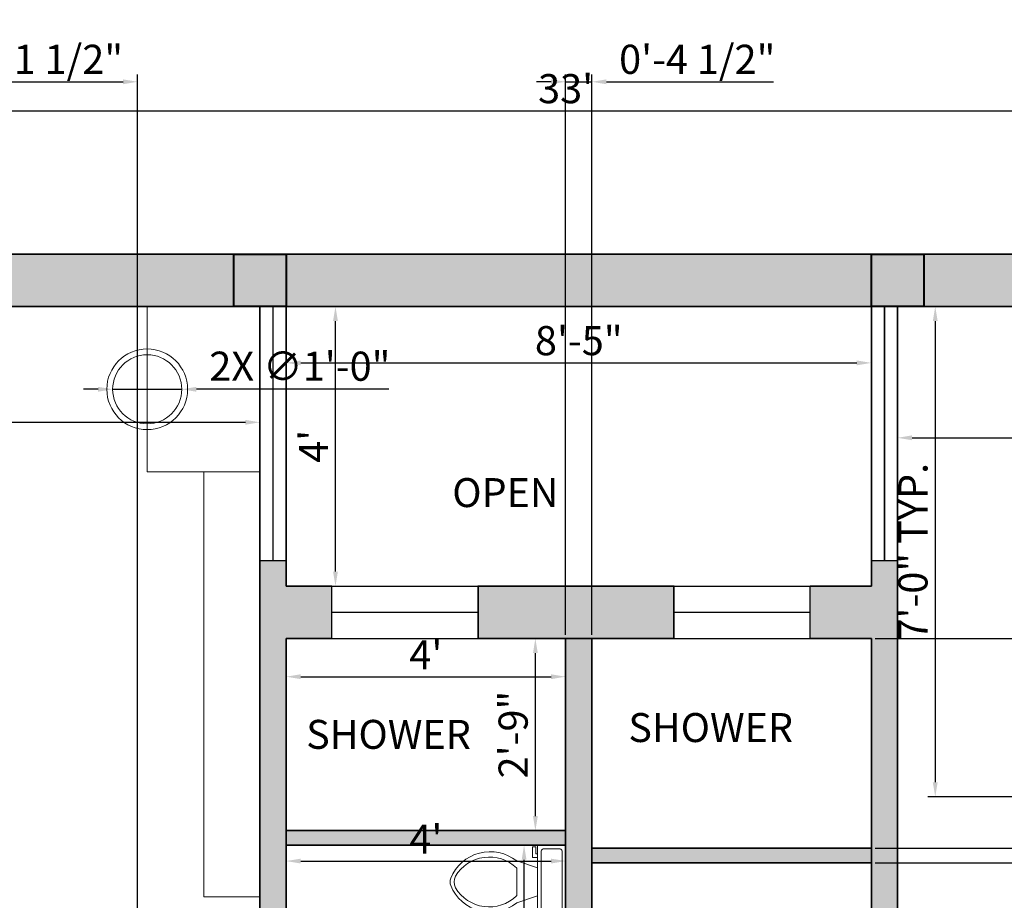
# Model space of a CAD drawing. Units: inches. Extents: x 1674 to 2231, y 1328 to 1959.
# Tile 5 of 6: x 1841 to 2010, y 1807 to 1959. Entities that reach past the tile are written whole.
import ezdxf

# ---------------------------------------------------------------- set-up
doc = ezdxf.new("R2010")
doc.units = ezdxf.units.IN
for name, color, linetype, lineweight in [('A-ANNO-DIMS', 113, 'Continuous', 18), ('A-AREA-IDEN', 113, 'Continuous', 18), ('A-COLS-PATT', 10, 'Continuous', 13), ('A-FLOR-CASE', 211, 'Continuous', 18), ('A-FLOR-FIXT', 211, 'Continuous', 18), ('A-WALL-PATT', 140, 'Continuous', 13), ('COLUMN', 10, 'Continuous', 40), ('FUR', 211, 'Continuous', 18), ('WALL', 7, 'Continuous', 35), ('WN', 181, 'Continuous', 25)]:
    doc.layers.add(name, color=color, linetype=linetype, lineweight=lineweight)
doc.styles.get("Standard").update_dxf_attribs({"font": 'arial.ttf'})
doc.dimstyles.new('ISO-25', dxfattribs={"dimtxt": 5, "dimasz": 2.5, "dimexe": 1.25, "dimexo": 0.625, "dimtad": 1, "dimdec": 0, "dimlunit": 4, "dimtxsty": 'Standard', "dimcen": 2.5, "dimadec": 0, "dimazin": 0, "dimtfac": 1, "dimtdec": 0, "dimtmove": 0, "dimatfit": 3, "dimfxl": 1, "dimarcsym": 0})

# ---------------------------------------------------------------- blocks, each defined once
blk = doc.blocks.new('*U4')
for p, q in [((9.5, -6), (9.5, -2)), ((-8, -8.5), (-8, -8)), ((-7, -8), (-7, -9.5)), ((-4, -8), (-6, -14)), ((4, -8), (6, -14)), ((-10, -8.5), (-8, -8.5)), ((-10, -9.5), (-10, -8.5)), ((-7, -9.5), (-10, -9.5)), ((4, -14), (-4, -14))]:
    blk.add_line(p, q)
blk.add_lwpolyline([(10.5, -8), (10.5, 0), (-10.5, 0), (-10.5, -8)], close=True)
for points in [[(-9.5, -2), (-9.5, -6)], [(8.5, -1), (-8.5, -1)], [(-8.5, -7), (8.5, -7)]]:
    blk.add_lwpolyline(points)
for centre, radius, start, end in [((-8.62, -1.88), 0.884, 81.8699, 188.1301), ((8.62, -1.88), 0.884, 351.8699, 98.1301), ((-8.62, -6.12), 0.884, 171.8699, 278.1301), ((8.62, -6.12), 0.884, 261.8699, 8.1301), ((3.52, -21.58), 12.17, 141.4691, 247.9714), ((4.2, -21.82), 11.33, 136.3677, 238.9468), ((-3.52, -21.58), 12.17, 292.0284, 38.5307), ((-4.2, -21.82), 11.33, 301.053, 43.6321), ((0, -27.88), 4, 245.7318, 294.2682), ((0, -29), 4, 254.8605, 285.1395)]:
    blk.add_arc(centre, radius, start, end)
blk = doc.blocks.new('*D9')
at = {"layer": 'A-ANNO-DIMS', "color": 0, "lineweight": -2, "transparency": 16777216}
for p, q in [((1736.27, 1918.98), (1736.27, 1944.21)), ((1738.77, 1942.96), (2129.77, 1942.96)), ((2132.27, 1918.98), (2132.27, 1944.21))]:
    blk.add_line(p, q, dxfattribs=at)
at = {"layer": 'A-ANNO-DIMS', "color": 0, "lineweight": 100, "transparency": 16777216}
for points in [[(1738.77, 1943.37), (1738.77, 1942.54), (1736.27, 1942.96)], [(2129.77, 1943.37), (2129.77, 1942.54), (2132.27, 1942.96)]]:
    blk.add_solid(points, dxfattribs=at)
at = {"layer": 'Defpoints', "color": 0, "lineweight": 100, "transparency": 16777216}
for p in [(2132.27, 1942.96), (1736.27, 1918.36), (2132.27, 1918.36)]:
    blk.add_point(p, dxfattribs=at)
at = {"layer": 'A-ANNO-DIMS', "color": 0, "transparency": 16777216, "insert": (1934.27, 1946.13), "char_height": 5, "attachment_point": 5}
blk.add_mtext("33'", dxfattribs=at)
blk = doc.blocks.new('*D11')
at = {"layer": 'A-ANNO-DIMS', "color": 0, "lineweight": -2, "transparency": 16777216}
for p, q in [((1745.27, 1908.73), (1745.27, 1888.23)), ((1881.77, 1908.73), (1881.77, 1888.23)), ((1747.77, 1889.48), (1879.27, 1889.48))]:
    blk.add_line(p, q, dxfattribs=at)
at = {"layer": 'A-ANNO-DIMS', "color": 0, "lineweight": 100, "transparency": 16777216}
for points in [[(1747.77, 1889.9), (1747.77, 1889.07), (1745.27, 1889.48)], [(1879.27, 1889.9), (1879.27, 1889.07), (1881.77, 1889.48)]]:
    blk.add_solid(points, dxfattribs=at)
at = {"layer": 'Defpoints', "color": 0, "lineweight": 100, "transparency": 16777216}
for p in [(1745.27, 1909.36), (1881.77, 1909.36), (1881.77, 1889.48)]:
    blk.add_point(p, dxfattribs=at)
at = {"layer": 'A-ANNO-DIMS', "color": 0, "transparency": 16777216, "insert": (1813.52, 1892.66), "char_height": 5, "attachment_point": 5}
blk.add_mtext('11\'-5"', dxfattribs=at)
blk = doc.blocks.new('*D13')
at = {"layer": 'A-ANNO-DIMS', "color": 0, "lineweight": -2, "transparency": 16777216}
for p, q in [((1886.27, 1908.73), (1886.27, 1898.44)), ((1986.77, 1908.73), (1986.77, 1898.44)), ((1888.77, 1899.69), (1984.27, 1899.69))]:
    blk.add_line(p, q, dxfattribs=at)
at = {"layer": 'A-ANNO-DIMS', "color": 0, "lineweight": 100, "transparency": 16777216}
for points in [[(1888.77, 1900.1), (1888.77, 1899.27), (1886.27, 1899.69)], [(1984.27, 1900.1), (1984.27, 1899.27), (1986.77, 1899.69)]]:
    blk.add_solid(points, dxfattribs=at)
at = {"layer": 'Defpoints', "color": 0, "lineweight": 100, "transparency": 16777216}
for p in [(1886.27, 1909.36), (1986.77, 1909.36), (1986.77, 1899.69)]:
    blk.add_point(p, dxfattribs=at)
at = {"layer": 'A-ANNO-DIMS', "color": 0, "transparency": 16777216, "insert": (1936.52, 1902.86), "char_height": 5, "attachment_point": 5}
blk.add_mtext('8\'-5"', dxfattribs=at)
blk = doc.blocks.new('*D14')
at = {"layer": 'A-ANNO-DIMS', "color": 0, "lineweight": -2, "transparency": 16777216}
for p, q in [((1886.9, 1909.36), (1895.99, 1909.36)), ((1894.74, 1863.86), (1894.74, 1906.86)), ((1886.9, 1861.36), (1895.99, 1861.36))]:
    blk.add_line(p, q, dxfattribs=at)
at = {"layer": 'A-ANNO-DIMS', "color": 0, "lineweight": 100, "transparency": 16777216}
for points in [[(1894.32, 1906.86), (1895.16, 1906.86), (1894.74, 1909.36)], [(1894.32, 1863.86), (1895.16, 1863.86), (1894.74, 1861.36)]]:
    blk.add_solid(points, dxfattribs=at)
at = {"layer": 'Defpoints', "color": 0, "lineweight": 100, "transparency": 16777216}
for p in [(1886.27, 1909.36), (1894.74, 1909.36), (1886.27, 1861.36)]:
    blk.add_point(p, dxfattribs=at)
at = {"layer": 'A-ANNO-DIMS', "color": 0, "transparency": 16777216, "insert": (1891.61, 1885.36), "char_height": 5, "attachment_point": 5, "rotation": 90}
blk.add_mtext("4'", dxfattribs=at)
blk = doc.blocks.new('*D15')
at = {"layer": 'A-ANNO-DIMS', "color": 0, "lineweight": -2, "transparency": 16777216}
for p, q in [((1886.27, 1851.73), (1886.27, 1844.55)), ((1934.27, 1851.73), (1934.27, 1844.55)), ((1888.77, 1845.8), (1931.77, 1845.8))]:
    blk.add_line(p, q, dxfattribs=at)
at = {"layer": 'A-ANNO-DIMS', "color": 0, "lineweight": 100, "transparency": 16777216}
for points in [[(1888.77, 1846.21), (1888.77, 1845.38), (1886.27, 1845.8)], [(1931.77, 1846.21), (1931.77, 1845.38), (1934.27, 1845.8)]]:
    blk.add_solid(points, dxfattribs=at)
at = {"layer": 'Defpoints', "color": 0, "lineweight": 100, "transparency": 16777216}
for p in [(1886.27, 1852.36), (1934.27, 1852.36), (1934.27, 1845.8)]:
    blk.add_point(p, dxfattribs=at)
at = {"layer": 'A-ANNO-DIMS', "color": 0, "transparency": 16777216, "insert": (1910.27, 1848.92), "char_height": 5, "attachment_point": 5}
blk.add_mtext("4'", dxfattribs=at)
blk = doc.blocks.new('*D16')
at = {"layer": 'A-ANNO-DIMS', "color": 0, "lineweight": -2, "transparency": 16777216}
for p, q in [((1933.65, 1852.36), (1927.82, 1852.36)), ((1929.07, 1821.86), (1929.07, 1849.86)), ((1933.65, 1819.36), (1927.82, 1819.36))]:
    blk.add_line(p, q, dxfattribs=at)
at = {"layer": 'A-ANNO-DIMS', "color": 0, "lineweight": 100, "transparency": 16777216}
for points in [[(1928.66, 1849.86), (1929.49, 1849.86), (1929.07, 1852.36)], [(1928.66, 1821.86), (1929.49, 1821.86), (1929.07, 1819.36)]]:
    blk.add_solid(points, dxfattribs=at)
at = {"layer": 'Defpoints', "color": 0, "lineweight": 100, "transparency": 16777216}
for p in [(1929.07, 1852.36), (1934.27, 1852.36), (1934.27, 1819.36)]:
    blk.add_point(p, dxfattribs=at)
at = {"layer": 'A-ANNO-DIMS', "color": 0, "transparency": 16777216, "insert": (1925.9, 1835.86), "char_height": 5, "attachment_point": 5, "rotation": 90}
blk.add_mtext('2\'-9"', dxfattribs=at)
blk = doc.blocks.new('*D17')
at = {"layer": 'A-ANNO-DIMS', "color": 0, "lineweight": -2, "transparency": 16777216}
for p, q in [((1886.27, 1816.23), (1886.27, 1812.89)), ((1934.27, 1816.23), (1934.27, 1812.89)), ((1888.77, 1814.14), (1931.77, 1814.14))]:
    blk.add_line(p, q, dxfattribs=at)
at = {"layer": 'A-ANNO-DIMS', "color": 0, "lineweight": 100, "transparency": 16777216}
for points in [[(1888.77, 1814.55), (1888.77, 1813.72), (1886.27, 1814.14)], [(1931.77, 1814.55), (1931.77, 1813.72), (1934.27, 1814.14)]]:
    blk.add_solid(points, dxfattribs=at)
at = {"layer": 'Defpoints', "color": 0, "lineweight": 100, "transparency": 16777216}
for p in [(1886.27, 1816.86), (1934.27, 1816.86), (1934.27, 1814.14)]:
    blk.add_point(p, dxfattribs=at)
at = {"layer": 'A-ANNO-DIMS', "color": 0, "transparency": 16777216, "insert": (1910.27, 1817.26), "char_height": 5, "attachment_point": 5}
blk.add_mtext("4'", dxfattribs=at)
blk = doc.blocks.new('*D18')
at = {"layer": 'A-ANNO-DIMS', "color": 0, "lineweight": -2, "transparency": 16777216}
for p, q in [((1933.65, 1816.86), (1925.88, 1816.86)), ((1927.13, 1779.86), (1927.13, 1814.36)), ((1933.65, 1777.36), (1925.88, 1777.36))]:
    blk.add_line(p, q, dxfattribs=at)
at = {"layer": 'A-ANNO-DIMS', "color": 0, "lineweight": 100, "transparency": 16777216}
for points in [[(1926.72, 1814.36), (1927.55, 1814.36), (1927.13, 1816.86)], [(1926.72, 1779.86), (1927.55, 1779.86), (1927.13, 1777.36)]]:
    blk.add_solid(points, dxfattribs=at)
at = {"layer": 'Defpoints', "color": 0, "lineweight": 100, "transparency": 16777216}
for p in [(1927.13, 1816.86), (1934.27, 1816.86), (1934.27, 1777.36)]:
    blk.add_point(p, dxfattribs=at)
at = {"layer": 'A-ANNO-DIMS', "color": 0, "transparency": 16777216, "insert": (1923.95, 1797.11), "char_height": 5, "attachment_point": 5, "rotation": 90}
blk.add_mtext('3\'-4"', dxfattribs=at)
blk = doc.blocks.new('*D19')
at = {"layer": 'A-ANNO-DIMS', "color": 0, "lineweight": -2, "transparency": 16777216}
for p, q in [((1991.27, 1908.73), (1991.27, 1885.57)), ((2123.27, 1908.73), (2123.27, 1885.57)), ((1993.77, 1886.82), (2120.77, 1886.82))]:
    blk.add_line(p, q, dxfattribs=at)
at = {"layer": 'A-ANNO-DIMS', "color": 0, "lineweight": 100, "transparency": 16777216}
for points in [[(1993.77, 1887.24), (1993.77, 1886.4), (1991.27, 1886.82)], [(2120.77, 1887.24), (2120.77, 1886.4), (2123.27, 1886.82)]]:
    blk.add_solid(points, dxfattribs=at)
at = {"layer": 'Defpoints', "color": 0, "lineweight": 100, "transparency": 16777216}
for p in [(1991.27, 1909.36), (2123.27, 1909.36), (2123.27, 1886.82)]:
    blk.add_point(p, dxfattribs=at)
at = {"layer": 'A-ANNO-DIMS', "color": 0, "transparency": 16777216, "insert": (2057.27, 1889.95), "char_height": 5, "attachment_point": 5}
blk.add_mtext("11'", dxfattribs=at)
blk = doc.blocks.new('STOOL-ROUND')
for radius in [6.93, 5.93]:
    blk.add_circle((6.93, 6.93), radius)
blk = doc.blocks.new('*D47')
at = {"layer": 'A-ANNO-DIMS', "color": 0, "lineweight": -2, "transparency": 16777216}
for p, q in [((2011.29, 1909.36), (1996.49, 1909.36)), ((1997.74, 1906.86), (1997.74, 1827.66)), ((2011.29, 1825.16), (1996.49, 1825.16))]:
    blk.add_line(p, q, dxfattribs=at)
at = {"layer": 'A-ANNO-DIMS', "color": 0, "lineweight": 100, "transparency": 16777216}
for points in [[(1997.32, 1906.86), (1998.16, 1906.86), (1997.74, 1909.36)], [(1997.32, 1827.66), (1998.16, 1827.66), (1997.74, 1825.16)]]:
    blk.add_solid(points, dxfattribs=at)
at = {"layer": 'Defpoints', "color": 0, "lineweight": 100, "transparency": 16777216}
for p in [(2011.91, 1909.36), (1997.74, 1825.16), (2011.91, 1825.16)]:
    blk.add_point(p, dxfattribs=at)
at = {"layer": 'A-ANNO-DIMS', "color": 0, "transparency": 16777216, "insert": (1994.56, 1867.26), "char_height": 5, "attachment_point": 5, "rotation": 90}
blk.add_mtext('7\'-0" TYP.', dxfattribs=at)
blk = doc.blocks.new('*D52')
at = {"layer": 'A-ANNO-DIMS', "color": 0, "lineweight": -2, "transparency": 16777216}
for p, q in [((1987.4, 1813.86), (2163.12, 1813.86)), ((2161.87, 1755.86), (2161.87, 1811.36)), ((1987.4, 1753.36), (2163.12, 1753.36))]:
    blk.add_line(p, q, dxfattribs=at)
at = {"layer": 'A-ANNO-DIMS', "color": 0, "lineweight": 100, "transparency": 16777216}
for points in [[(2161.45, 1811.36), (2162.29, 1811.36), (2161.87, 1813.86)], [(2161.45, 1755.86), (2162.29, 1755.86), (2161.87, 1753.36)]]:
    blk.add_solid(points, dxfattribs=at)
at = {"layer": 'Defpoints', "color": 0, "lineweight": 100, "transparency": 16777216}
for p in [(1986.77, 1813.86), (2161.87, 1813.86), (1986.77, 1753.36)]:
    blk.add_point(p, dxfattribs=at)
at = {"layer": 'A-ANNO-DIMS', "color": 0, "transparency": 16777216, "insert": (2158.66, 1783.61), "char_height": 5, "attachment_point": 5, "rotation": 90}
blk.add_mtext('5\'-0 1/2"', dxfattribs=at)
blk = doc.blocks.new('*D53')
at = {"layer": 'A-ANNO-DIMS', "color": 0, "lineweight": -2, "transparency": 16777216}
for p, q in [((1987.4, 1852.36), (2163.12, 1852.36)), ((2161.87, 1818.86), (2161.87, 1849.86)), ((1987.4, 1816.36), (2163.12, 1816.36))]:
    blk.add_line(p, q, dxfattribs=at)
at = {"layer": 'A-ANNO-DIMS', "color": 0, "lineweight": 100, "transparency": 16777216}
for points in [[(2161.45, 1849.86), (2162.29, 1849.86), (2161.87, 1852.36)], [(2161.45, 1818.86), (2162.29, 1818.86), (2161.87, 1816.36)]]:
    blk.add_solid(points, dxfattribs=at)
at = {"layer": 'Defpoints', "color": 0, "lineweight": 100, "transparency": 16777216}
for p in [(1986.77, 1852.36), (2161.87, 1852.36), (1986.77, 1816.36)]:
    blk.add_point(p, dxfattribs=at)
at = {"layer": 'A-ANNO-DIMS', "color": 0, "transparency": 16777216, "insert": (2158.69, 1834.36), "char_height": 5, "attachment_point": 5, "rotation": 90}
blk.add_mtext('3\'-0"', dxfattribs=at)
blk = doc.blocks.new('*D56')
at = {"layer": 'A-ANNO-DIMS', "color": 0, "lineweight": -2, "transparency": 16777216}
for p, q in [((1825.14, 1600.98), (1825.14, 1949.21)), ((1827.64, 1947.96), (1858.27, 1947.96)), ((1860.77, 1600.98), (1860.77, 1949.21))]:
    blk.add_line(p, q, dxfattribs=at)
at = {"layer": 'A-ANNO-DIMS', "color": 0, "lineweight": 100, "transparency": 16777216}
for points in [[(1827.64, 1948.37), (1827.64, 1947.54), (1825.14, 1947.96)], [(1858.27, 1948.37), (1858.27, 1947.54), (1860.77, 1947.96)]]:
    blk.add_solid(points, dxfattribs=at)
at = {"layer": 'Defpoints', "color": 0, "lineweight": 100, "transparency": 16777216}
for p in [(1860.77, 1947.96), (1825.14, 1600.36), (1860.77, 1600.36)]:
    blk.add_point(p, dxfattribs=at)
at = {"layer": 'A-ANNO-DIMS', "color": 0, "transparency": 16777216, "insert": (1842.96, 1951.17), "char_height": 5, "attachment_point": 5}
blk.add_mtext('2\'-11 1/2"', dxfattribs=at)
blk = doc.blocks.new('*D57')
at = {"layer": 'A-ANNO-DIMS', "color": 0, "lineweight": -2, "transparency": 16777216}
for p, q in [((1931.77, 1947.96), (1929.27, 1947.96)), ((1934.27, 1852.98), (1934.27, 1949.21)), ((1934.27, 1947.96), (1938.77, 1947.96)), ((1938.77, 1852.98), (1938.77, 1949.21)), ((1941.27, 1947.96), (1969.96, 1947.96))]:
    blk.add_line(p, q, dxfattribs=at)
at = {"layer": 'A-ANNO-DIMS', "color": 0, "lineweight": 100, "transparency": 16777216}
for points in [[(1931.77, 1948.37), (1931.77, 1947.54), (1934.27, 1947.96)], [(1941.27, 1948.37), (1941.27, 1947.54), (1938.77, 1947.96)]]:
    blk.add_solid(points, dxfattribs=at)
at = {"layer": 'Defpoints', "color": 0, "lineweight": 100, "transparency": 16777216}
for p in [(1938.77, 1947.96), (1934.27, 1852.36), (1938.77, 1852.36)]:
    blk.add_point(p, dxfattribs=at)
at = {"layer": 'A-ANNO-DIMS', "color": 0, "transparency": 16777216, "insert": (1956.87, 1951.17), "char_height": 5, "attachment_point": 5}
blk.add_mtext('0\'-4 1/2"', dxfattribs=at)
blk = doc.blocks.new('*D60')
at = {"layer": 'A-ANNO-DIMS', "color": 0, "lineweight": -2, "transparency": 16777216}
for p, q in [((1853.98, 1895.16), (1851.48, 1895.16)), ((1856.48, 1895.16), (1868.35, 1895.15)), ((1903.9, 1895.15), (1870.85, 1895.15))]:
    blk.add_line(p, q, dxfattribs=at)
at = {"layer": 'A-ANNO-DIMS', "color": 0, "lineweight": 100, "transparency": 16777216}
for points in [[(1853.98, 1895.57), (1853.98, 1894.74), (1856.48, 1895.16)], [(1870.85, 1895.57), (1870.85, 1894.74), (1868.35, 1895.15)]]:
    blk.add_solid(points, dxfattribs=at)
at = {"layer": 'Defpoints', "color": 0, "lineweight": 100, "transparency": 16777216}
for p in [(1856.48, 1895.16), (1868.35, 1895.15)]:
    blk.add_point(p, dxfattribs=at)
at = {"layer": 'A-ANNO-DIMS', "color": 0, "transparency": 16777216, "insert": (1888.63, 1898.47), "char_height": 5, "attachment_point": 5, "rotation": 359.9954}
blk.add_mtext('2X ∅1\'-0"', dxfattribs=at)

msp = doc.modelspace()

# ---------------------------------------------------------------- hatches: boundary and pattern name
at = {"layer": 'A-COLS-PATT'}
h = msp.add_hatch(color=256, dxfattribs=at)
h.dxf.hatch_style = 1
h.paths.add_polyline_path([(1745.27, 1918.36), (1736.27, 1918.36), (1736.27, 1909.36), (1745.27, 1909.36)])
h.paths.add_polyline_path([(1886.27, 1918.36), (1877.27, 1918.36), (1877.27, 1909.36), (1886.27, 1909.36)])
h.paths.add_polyline_path([(1995.77, 1918.36), (1986.77, 1918.36), (1986.77, 1909.36), (1995.77, 1909.36)])
h.paths.add_polyline_path([(2132.27, 1918.36), (2123.27, 1918.36), (2123.27, 1909.36), (2132.27, 1909.36)])
h.paths.add_polyline_path([(1745.27, 1757.86), (1736.27, 1757.86), (1736.27, 1748.86), (1745.27, 1748.86)])
h.paths.add_polyline_path([(1886.27, 1757.86), (1877.27, 1757.86), (1877.27, 1748.86), (1886.27, 1748.86)])
h.paths.add_polyline_path([(2132.27, 1757.81), (2123.27, 1757.81), (2123.27, 1748.81), (2132.27, 1748.81)])
h.paths.add_polyline_path([(1995.77, 1757.86), (1986.77, 1757.86), (1986.77, 1748.86), (1995.77, 1748.86)])
h.paths.add_polyline_path([(2132.27, 1625.36), (2123.27, 1625.36), (2123.27, 1616.36), (2132.27, 1616.36)])
h.paths.add_polyline_path([(1995.77, 1625.36), (1986.77, 1625.36), (1986.77, 1616.36), (1995.77, 1616.36)])
h.paths.add_polyline_path([(1869.77, 1604.86), (1860.77, 1604.86), (1860.77, 1595.86), (1869.77, 1595.86)])
h.paths.add_polyline_path([(1745.27, 1609.36), (1736.27, 1609.36), (1736.27, 1600.36), (1745.27, 1600.36)])
h.paths.add_polyline_path([(1745.27, 1504.36), (1736.27, 1504.36), (1736.27, 1495.36), (1745.27, 1495.36)])
h.paths.add_polyline_path([(1870.95, 1504.36), (1861.95, 1504.36), (1861.95, 1495.36), (1870.95, 1495.36)])
h.paths.add_polyline_path([(1995.77, 1504.36), (1986.77, 1504.36), (1986.77, 1495.36), (1995.77, 1495.36)])
h.paths.add_polyline_path([(1995.77, 1447.36), (1986.77, 1447.36), (1986.77, 1438.36), (1995.77, 1438.36)])
h.paths.add_polyline_path([(2132.27, 1447.36), (2123.27, 1447.36), (2123.27, 1438.36), (2132.27, 1438.36)])
at = {"layer": 'A-WALL-PATT'}
h = msp.add_hatch(color=256, dxfattribs=at)
h.dxf.hatch_style = 1
h.paths.add_polyline_path([(1877.27, 1918.36), (1745.27, 1918.36), (1745.27, 1909.36), (1877.27, 1909.36)])
h.paths.add_polyline_path([(1986.77, 1918.36), (1886.27, 1918.36), (1886.27, 1909.36), (1986.77, 1909.36)])
h.paths.add_polyline_path([(2123.27, 1918.36), (1995.77, 1918.36), (1995.77, 1909.36), (2123.27, 1909.36)])
h.paths.add_polyline_path([(1894.11, 1861.36), (1886.27, 1861.36), (1886.27, 1865.74), (1881.77, 1865.74), (1881.77, 1808), (1881.77, 1798.89), (1884.87, 1798.89, -0.017002), (1886.27, 1798.84), (1886.27, 1852.36), (1894.11, 1852.36)])
h.paths.add_polyline_path([(1952.87, 1861.36), (1919.24, 1861.36), (1919.24, 1852.36), (1952.87, 1852.36)])
h.paths.add_polyline_path([(1991.27, 1865.74), (1986.77, 1865.74), (1986.77, 1861.36), (1976.26, 1861.36), (1976.26, 1852.36), (1986.77, 1852.36), (1986.77, 1847.49), (1986.77, 1757.86), (1991.27, 1757.86), (1991.27, 1852.36)])
h.paths.add_polyline_path([(1986.77, 1816.36), (1938.77, 1816.36), (1938.77, 1813.86), (1986.77, 1813.86)])
h.paths.add_polyline_path([(1934.27, 1819.36), (1886.27, 1819.36), (1886.27, 1816.86), (1934.27, 1816.86)])
h.paths.add_polyline_path([(1938.77, 1852.36), (1934.27, 1852.36), (1934.27, 1753.36), (1934.27, 1748.86), (1938.77, 1748.86), (1938.77, 1753.36)])
h.paths.add_polyline_path([(1934.27, 1777.36), (1915.46, 1777.36), (1886.27, 1777.36), (1886.27, 1772.86), (1934.27, 1772.86)])
h.paths.add_polyline_path([(1986.77, 1753.36), (1967.96, 1753.36), (1961.77, 1753.36, -0.017002), (1961.81, 1751.95), (1961.81, 1748.86), (1986.77, 1748.86)])
h.paths.add_polyline_path([(2000.84, 1753.36), (1995.77, 1753.36), (1995.77, 1748.86), (2000.84, 1748.86)])
h.paths.add_polyline_path([(1941.17, 1751.95), (1941.17, 1753.36), (1938.77, 1753.36), (1938.77, 1748.86), (1941.17, 1748.86)])
h.paths.add_polyline_path([(1877.27, 1753.36), (1875.49, 1753.36), (1875.49, 1748.86), (1877.27, 1748.86)])
h.paths.add_polyline_path([(1745.27, 1909.36), (1736.27, 1909.36), (1736.27, 1757.86), (1745.27, 1757.86), (1745.27, 1773.01)])
h.paths.add_polyline_path([(1778.41, 1645.36), (1745.27, 1645.36), (1745.27, 1640.86), (1778.41, 1640.86)])
h.paths.add_polyline_path([(1821.77, 1645.36), (1821.77, 1668.45), (1817.27, 1668.45), (1817.27, 1645.36), (1817.27, 1640.86), (1821.77, 1640.86)])
h.paths.add_polyline_path([(1817.27, 1645.36), (1813.39, 1645.36), (1813.39, 1640.86), (1817.27, 1640.86)])
h.paths.add_polyline_path([(1821.77, 1640.86), (1817.27, 1640.86), (1817.27, 1604.86), (1817.27, 1600.36), (1821.77, 1600.36)])
h.paths.add_polyline_path([(1825.14, 1604.86), (1821.77, 1604.86), (1821.77, 1600.36), (1825.14, 1600.36)])
h.paths.add_polyline_path([(1781.27, 1604.86), (1745.27, 1604.86), (1745.27, 1600.36), (1781.27, 1600.36)])
h = msp.add_hatch(color=256, dxfattribs=at)
h.dxf.hatch_style = 1
h.paths.add_polyline_path([(2132.27, 1909.36), (2123.27, 1909.36), (2123.27, 1757.81), (2132.27, 1757.81)], flags=17)
h.paths.add_polyline_path([(2123.27, 1753.36), (2040.84, 1753.36), (2040.84, 1748.86), (2123.27, 1748.86)], flags=17)
h.paths.add_polyline_path([(1840.51, 1753.36), (1745.27, 1753.36), (1745.27, 1748.86), (1817.27, 1748.86), (1840.51, 1748.86)], flags=17)
h.paths.add_polyline_path([(1745.27, 1748.86), (1736.27, 1748.86), (1736.27, 1609.36), (1745.27, 1609.36), (1745.27, 1640.86)], flags=17)
h.paths.add_polyline_path([(1745.27, 1600.36), (1736.27, 1600.36), (1736.27, 1504.36), (1745.27, 1504.36)], flags=17)
h.paths.add_polyline_path([(1745.27, 1495.36), (1736.27, 1495.36), (1736.27, 1447.36), (1745.27, 1447.36)], flags=17)
h.paths.add_polyline_path([(1820.35, 1504.36), (1787.69, 1504.36), (1787.69, 1495.36), (1820.35, 1495.36)], flags=17)
h.paths.add_polyline_path([(1750.58, 1504.36), (1745.27, 1504.36), (1745.27, 1495.36), (1750.58, 1495.36)], flags=17)
h.paths.add_polyline_path([(1861.95, 1504.36), (1857.47, 1504.36), (1857.47, 1495.36), (1861.95, 1495.36)], flags=17)
h.paths.add_polyline_path([(1873.66, 1504.36), (1870.95, 1504.36), (1870.95, 1495.36), (1873.66, 1495.36)], flags=17)
h.paths.add_polyline_path([(1900.85, 1501.36), (1900.85, 1504.36), (1895.88, 1504.36), (1895.88, 1495.36), (1900.85, 1495.36)], flags=17)
h.paths.add_polyline_path([(1869.77, 1595.86), (1865.27, 1595.86), (1865.27, 1504.36), (1869.77, 1504.36)], flags=17)
h.paths.add_polyline_path([(1958.26, 1504.36), (1940.74, 1504.36, -0.01877), (1940.85, 1501.36), (1940.85, 1495.36), (1958.26, 1495.36)], flags=17)
h.paths.add_polyline_path([(1995.77, 1531.51), (1986.77, 1531.51), (1986.77, 1504.36), (1995.77, 1504.36)], flags=17)
h.paths.add_polyline_path([(1986.77, 1504.36), (1980.49, 1504.36), (1980.49, 1495.36), (1986.77, 1495.36)], flags=17)
h.paths.add_polyline_path([(1995.77, 1616.36), (1986.77, 1616.36), (1986.77, 1585.02), (1995.77, 1585.02)], flags=17)
h.paths.add_polyline_path([(2000.1, 1620.86), (1995.77, 1620.86), (1995.77, 1616.36), (2000.1, 1616.36)], flags=17)
h.paths.add_polyline_path([(2053.57, 1620.86), (2040.1, 1620.86), (2040.1, 1616.36), (2053.57, 1616.36)], flags=17)
h.paths.add_polyline_path([(2123.27, 1620.86), (2109.12, 1620.86), (2109.12, 1616.36), (2123.27, 1616.36)], flags=17)
h.paths.add_polyline_path([(2132.27, 1616.36), (2123.27, 1616.36), (2123.27, 1447.36), (2132.27, 1447.36)], flags=17)
h.paths.add_polyline_path([(1986.77, 1447.36), (1870.95, 1447.36), (1870.95, 1438.36), (1986.77, 1438.36)])
h.paths.add_polyline_path([(1861.95, 1447.36), (1745.27, 1447.36), (1745.27, 1438.36), (1861.95, 1438.36)])
h.paths.add_polyline_path([(2132.27, 1918.36), (1736.27, 1918.36), (1736.27, 1504.36), (1745.27, 1504.36), (1745.27, 1600.36), (1745.27, 1909.36), (2123.27, 1909.36), (2123.27, 1447.36), (2132.27, 1447.36)])
h = msp.add_hatch(color=256, dxfattribs=at)
h.dxf.hatch_style = 1
h.paths.add_polyline_path([(1886.27, 1777.36), (1886.27, 1778.24), (1884.87, 1778.24), (1881.77, 1778.24), (1881.77, 1757.86), (1886.27, 1757.86)], flags=17)
h.paths.add_polyline_path([(2132.27, 1918.36), (1736.27, 1918.36), (1736.27, 1757.86), (1745.27, 1757.86), (1745.27, 1773.01), (1745.27, 1909.36), (2123.27, 1909.36), (2123.27, 1757.81), (2132.27, 1757.81)])

# ---------------------------------------------------------------- linework, layer by layer
at = {"layer": 'A-FLOR-CASE'}
for points in [[(1881.77, 1909.36), (1862.42, 1909.36), (1862.42, 1880.96), (1881.77, 1880.96)], [(1881.77, 1880.96), (1872.11, 1880.96), (1872.11, 1808), (1881.77, 1808)]]:
    msp.add_lwpolyline(points, close=True, dxfattribs=at)
at = {"layer": 'COLUMN'}
for points in [[(1877.27, 1918.36), (1886.27, 1918.36), (1886.27, 1909.36), (1877.27, 1909.36)], [(1986.77, 1918.36), (1995.77, 1918.36), (1995.77, 1909.36), (1986.77, 1909.36)]]:
    msp.add_lwpolyline(points, close=True, dxfattribs=at)
at = {"layer": 'WALL'}
for p, q in [((1736.27, 1918.36), (2132.27, 1918.36)), ((1745.27, 1909.36), (1881.77, 1909.36)), ((1881.77, 1909.36), (1881.77, 1798.89)), ((1886.27, 1909.36), (1886.27, 1861.36)), ((1886.27, 1909.36), (1986.77, 1909.36)), ((1986.77, 1909.36), (1986.77, 1861.36)), ((1991.27, 1909.36), (1991.27, 1852.36)), ((1894.11, 1861.36), (1886.27, 1861.36)), ((1952.87, 1861.36), (1919.24, 1861.36)), ((1986.77, 1861.36), (1976.26, 1861.36)), ((1886.27, 1852.36), (1894.11, 1852.36)), ((1886.27, 1852.36), (1886.27, 1798.84)), ((1894.11, 1852.36), (1886.27, 1852.36)), ((1919.24, 1852.36), (1934.27, 1852.36)), ((1952.87, 1852.36), (1919.24, 1852.36)), ((1934.27, 1852.36), (1934.27, 1819.36)), ((1934.27, 1852.36), (1934.27, 1753.36)), ((1938.77, 1852.36), (1938.77, 1753.36)), ((1938.77, 1852.36), (1938.77, 1816.36)), ((1986.77, 1852.36), (1976.26, 1852.36)), ((1986.77, 1852.36), (1986.77, 1753.36)), ((1986.77, 1852.36), (1986.77, 1847.49)), ((1991.27, 1852.36), (1991.27, 1757.86)), ((1934.27, 1819.36), (1886.27, 1819.36)), ((1934.27, 1819.36), (1934.27, 1753.36)), ((1934.27, 1816.86), (1886.27, 1816.86)), ((1938.77, 1816.36), (1986.77, 1816.36)), ((1938.77, 1813.86), (1986.77, 1813.86))]:
    msp.add_line(p, q, dxfattribs=at)
for points in [[(1995.77, 1438.36), (1736.27, 1438.36), (1736.27, 1918.36), (2132.27, 1918.36), (2132.27, 1438.36), (2123.27, 1438.36)], [(1995.77, 1447.36), (1745.27, 1447.36), (1745.27, 1909.36), (2123.27, 1909.36), (2123.27, 1447.36)]]:
    msp.add_lwpolyline(points, dxfattribs=at)
msp.add_lwpolyline([(1919.24, 1852.36), (1952.87, 1852.36), (1952.87, 1861.36), (1919.24, 1861.36)], close=True, dxfattribs=at)
at = {"layer": 'WN'}
for p, q in [((1881.77, 1909.36), (1881.77, 1865.74)), ((1884.02, 1865.74), (1884.02, 1909.36)), ((1886.27, 1909.36), (1886.27, 1865.74)), ((1989.02, 1865.74), (1989.02, 1909.36)), ((1989.02, 1909.36), (1989.02, 1865.74)), ((1881.77, 1865.74), (1886.27, 1865.74)), ((1986.77, 1865.74), (1991.27, 1865.74)), ((1894.11, 1852.36), (1894.11, 1861.36)), ((1894.11, 1861.36), (1919.24, 1861.36)), ((1919.24, 1852.36), (1919.24, 1861.36)), ((1952.87, 1852.36), (1952.87, 1861.36)), ((1952.87, 1861.36), (1976.26, 1861.36)), ((1976.26, 1852.36), (1976.26, 1861.36)), ((1894.11, 1856.86), (1919.24, 1856.86)), ((1952.87, 1856.86), (1976.26, 1856.86)), ((1894.11, 1852.36), (1919.24, 1852.36)), ((1952.87, 1852.36), (1976.26, 1852.36))]:
    msp.add_line(p, q, dxfattribs=at)
msp.add_lwpolyline([(1986.77, 1865.74), (1991.27, 1865.74), (1991.27, 1909.36), (1986.77, 1909.36)], close=True, dxfattribs=at)

# ---------------------------------------------------------------- block references
at = {"layer": 'A-FLOR-FIXT', "xscale": 0.6007383453482145, "yscale": 0.6007383453482145, "zscale": 0.6007383453482145, "rotation": 270}
msp.add_blockref('*U4', (1934.27, 1810.55), dxfattribs=at)
at = {"layer": 'FUR'}
msp.add_blockref('STOOL-ROUND', (1855.48, 1888.22), dxfattribs=at)

# ---------------------------------------------------------------- texts
at = {"layer": 'A-AREA-IDEN', "char_height": 4.973, "attachment_point": 1}
for s, insert in [('OPEN', (1914.8, 1879.9)), ('SHOWER', (1889.71, 1838.38)), ('SHOWER', (1945.04, 1839.55))]:
    msp.add_mtext_dynamic_manual_height_columns(s, width=89.7127, gutter_width=24.87, heights=[0], dxfattribs=dict(at, insert=insert))

# ---------------------------------------------------------------- dimensions: what is measured, and where the dimension line sits
at = {"layer": 'A-ANNO-DIMS'}
for base, p1, p2, override, picture, middle in [((1860.77, 1947.96), (1825.14, 1600.36), (1860.77, 1600.36), {"dimdec": 1, "dimlfac": 1, "dimrnd": 0, "dimzin": 1, "dimdsep": 46, "dimlunit": 4, "dimfrac": 2}, '*D56', (1842.96, 1951.17)), ((1938.77, 1947.96), (1934.27, 1852.36), (1938.77, 1852.36), {"dimdec": 1, "dimlfac": 1, "dimrnd": 0, "dimzin": 1, "dimdsep": 46, "dimlunit": 4, "dimfrac": 2}, '*D57', (1956.87, 1951.17)), ((2132.27, 1942.96), (1736.27, 1918.36), (2132.27, 1918.36), {"dimclrd": 0, "dimclre": 0, "dimclrt": 0}, '*D9', (1934.27, 1946.13)), ((1881.77109151, 1889.48404083), (1745.27109151, 1909.35548105), (1881.77109151, 1909.35548105), {"dimclrd": 0, "dimclre": 0, "dimclrt": 0}, '*D11', (1813.52109151, 1892.66190577)), ((1986.77109151, 1899.68521907), (1886.27109151, 1909.35548105), (1986.77109151, 1909.35548105), {"dimclrd": 0, "dimclre": 0, "dimclrt": 0}, '*D13', (1936.52109151, 1902.86308401)), ((2123.27, 1886.82), (1991.27, 1909.36), (2123.27, 1909.36), {"dimclrd": 0, "dimclre": 0, "dimclrt": 0}, '*D19', (2057.27, 1889.95)), ((1934.27, 1845.8), (1886.27, 1852.36), (1934.27, 1852.36), {"dimclrd": 0, "dimclre": 0, "dimclrt": 0}, '*D15', (1910.27, 1848.92)), ((1934.27, 1814.14), (1886.27, 1816.86), (1934.27, 1816.86), {"dimclrd": 0, "dimclre": 0, "dimclrt": 0}, '*D17', (1910.27, 1817.26))]:
    dim = msp.add_linear_dim(base=base, p1=p1, p2=p2, dimstyle='ISO-25', override=override, dxfattribs=at)
    dim.commit()
    dim.dimension.update_dxf_attribs({"geometry": picture, "text_midpoint": middle})
for base, p1, p2, override, picture, middle in [((1894.74, 1909.36), (1886.27, 1861.36), (1886.27, 1909.36), {"dimclrd": 0, "dimclre": 0, "dimclrt": 0}, '*D14', (1891.61, 1885.36)), ((1929.07, 1852.36), (1934.27, 1819.36), (1934.27, 1852.36), {"dimclrd": 0, "dimclre": 0, "dimclrt": 0}, '*D16', (1925.9, 1835.86)), ((2161.87, 1852.36), (1986.77, 1816.36), (1986.77, 1852.36), {"dimdec": 1, "dimlfac": 1, "dimrnd": 0, "dimzin": 1, "dimdsep": 46, "dimlunit": 4, "dimfrac": 2}, '*D53', (2158.69, 1834.36)), ((1927.13363559, 1816.85548105), (1934.27109151, 1777.35548105), (1934.27109151, 1816.85548105), {"dimclrd": 0, "dimclre": 0, "dimclrt": 0}, '*D18', (1923.95406533, 1797.10548105)), ((2161.87, 1813.86), (1986.77, 1753.36), (1986.77, 1813.86), {"dimdec": 1, "dimlfac": 1, "dimrnd": 0, "dimzin": 1, "dimdsep": 46, "dimlunit": 4, "dimfrac": 2}, '*D52', (2158.66, 1783.61))]:
    dim = msp.add_linear_dim(base=base, p1=p1, p2=p2, angle=90, dimstyle='ISO-25', override=override, dxfattribs=at)
    dim.commit()
    dim.dimension.update_dxf_attribs({"geometry": picture, "text_midpoint": middle})
dim = msp.add_linear_dim(base=(1997.74, 1825.16), p1=(2011.91, 1909.36), p2=(2011.91, 1825.16), angle=270, text='<> TYP.', dimstyle='ISO-25', override={"dimdec": 1, "dimlfac": 1, "dimrnd": 0, "dimzin": 1, "dimdsep": 46, "dimlunit": 4, "dimfrac": 2}, dxfattribs=at)
dim.commit()
dim.dimension.update_dxf_attribs({"geometry": '*D47', "text_midpoint": (1994.56, 1867.26)})
dim = msp.add_diameter_dim_2p(p1=(1856.48, 1895.16), p2=(1868.35, 1895.15), text='2X <>', dimstyle='ISO-25', override={"dimdec": 1, "dimlfac": 1, "dimrnd": 0, "dimzin": 1, "dimdsep": 46, "dimlunit": 4, "dimfrac": 2}, dxfattribs=at)
dim.commit()
dim.dimension.update_dxf_attribs({"geometry": '*D60', "text_midpoint": (1888.62, 1895.15)})

doc.saveas('drawing.dxf')
